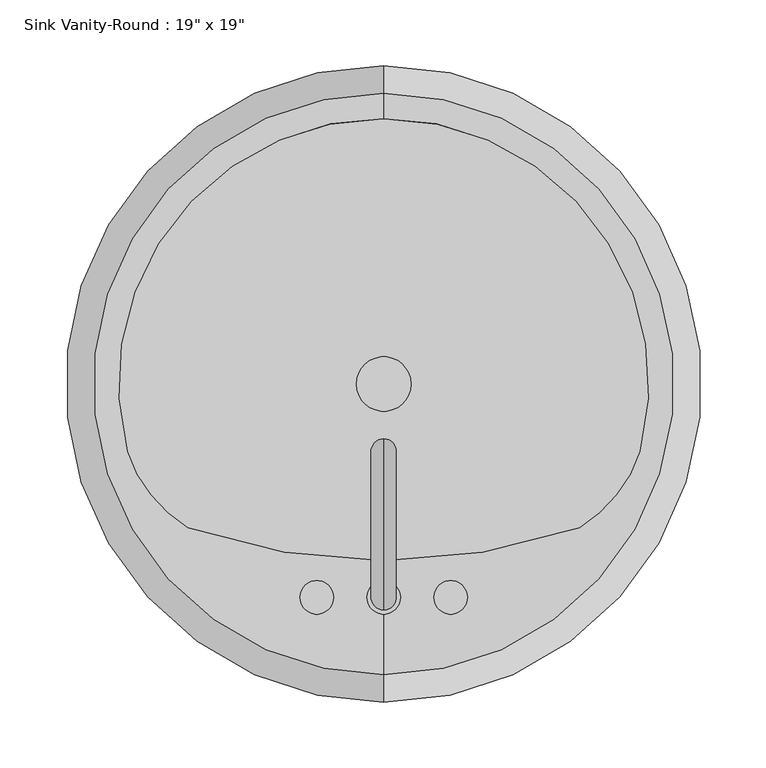
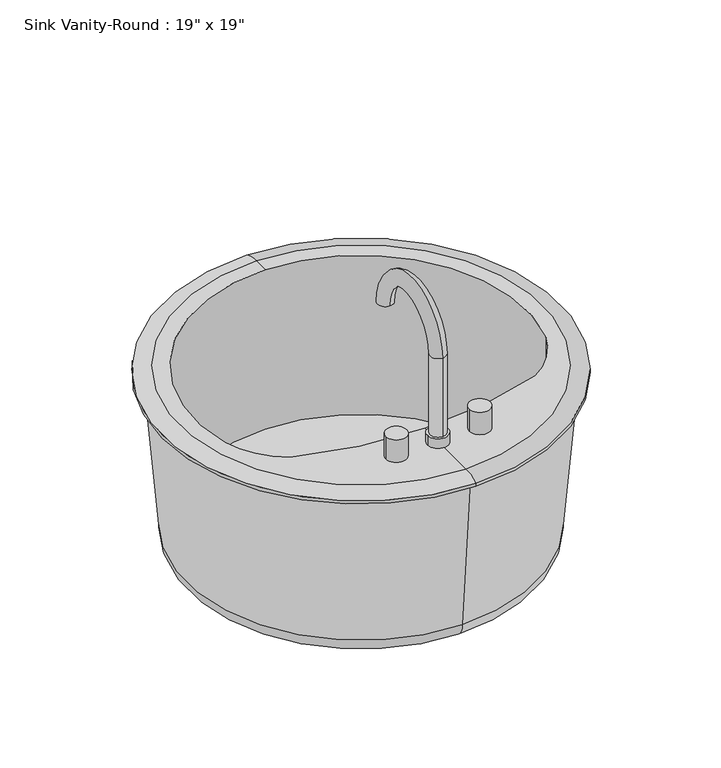
"""IFC4 building model written with IfcOpenShell, lengths in millimetres: flow terminal geometry."""

from ifc_helpers import new_model, si_unit, point, frame, frame_2d, origin, place, context, project, spatial, polyline, circle_curve, ellipse_curve, trimmed, segment, composite_curve, outline, extrude, source, transform, mapped, element, save
from ifc_brep_helpers import plane_surface, cylinder_surface, revolved_surface, advanced_brep


def flow_terminal_951b6bfb(model_context):
    return source(origin(), model_context, "Body", "SolidModel", [
        advanced_brep(
        [(83.9517406, -247.0927185, 796.925), (109.3517406, -247.0927185, 796.925), (96.6517406, -237.5677185, 909.6375), (96.6517406, -237.5677185, 809.1602909), (96.6517406, -256.6177185, 809.1602909), (96.6517406, -256.6177185, 909.6375), (96.6517406, -145.7775038, 909.6375), (96.6517406, -126.7275038, 909.6375), (83.9517406, -247.0927185, 809.1602909), (109.3517406, -247.0927185, 809.1602909)],
        [
            (0, 1, circle_curve(frame((96.6517406, -247.0927185, 796.925), z_axis=(0.0, 0.0, -1.0), x_axis=(1.0, 0.0, 0.0)), 12.7)),
            (1, 0, circle_curve(frame((96.6517406, -247.0927185, 796.925), z_axis=(0.0, 0.0, -1.0), x_axis=(1.0, 0.0, 0.0)), 12.7)),
            (2, 3),
            (3, 4, circle_curve(frame((96.6517406, -247.0927185, 809.1602909), z_axis=(0.0, 0.0, 1.0), x_axis=(0.0, -1.0, 0.0)), 9.525)),
            (4, 5),
            (5, 2, circle_curve(frame((96.6517406, -247.0927185, 909.6375), z_axis=(0.0, 0.0, -1.0), x_axis=(0.0, -1.0, 0.0)), 9.525)),
            (4, 3, circle_curve(frame((96.6517406, -247.0927185, 809.1602909), z_axis=(0.0, 0.0, 1.0), x_axis=(0.0, -1.0, 0.0)), 9.525)),
            (2, 5, circle_curve(frame((96.6517406, -247.0927185, 909.6375), z_axis=(0.0, 0.0, -1.0), x_axis=(0.0, -1.0, 0.0)), 9.525)),
            (6, 7, circle_curve(frame((96.6517406, -136.2525038, 909.6375), z_axis=(0.0, 0.0, -1.0), x_axis=(0.0, 1.0, 0.0)), 9.525)),
            (7, 6, circle_curve(frame((96.6517406, -136.2525038, 909.6375), z_axis=(0.0, 0.0, -1.0), x_axis=(0.0, 1.0, 0.0)), 9.525)),
            (5, 7, circle_curve(frame((96.6517406, -191.6726112, 909.6375), z_axis=(-1.0, 0.0, 0.0), x_axis=(0.0, -1.0, 0.0)), 64.9451073)),
            (6, 2, circle_curve(frame((96.6517406, -191.6726112, 909.6375), z_axis=(1.0, 0.0, 0.0), x_axis=(0.0, -1.0, 0.0)), 45.8951073)),
            (8, 9, circle_curve(frame((96.6517406, -247.0927185, 809.1602909), z_axis=(0.0, 0.0, 1.0), x_axis=(1.0, 0.0, 0.0)), 12.7)),
            (9, 8, circle_curve(frame((96.6517406, -247.0927185, 809.1602909), z_axis=(0.0, 0.0, 1.0), x_axis=(1.0, 0.0, 0.0)), 12.7)),
            (9, 1),
            (0, 8),
        ],
        [
            plane_surface(frame((96.6517406, -237.5677185, 796.925), z_axis=(0.0, 0.0, -1.0), x_axis=(1.0, 0.0, 0.0))),
            cylinder_surface(frame((96.6517406, -247.0927185, 796.925), z_axis=(0.0, 0.0, -1.0), x_axis=(0.0, -1.0, 0.0)), 9.525),
            plane_surface(frame((96.6517406, -191.6726112, 909.6375), z_axis=(0.0, 0.0, -1.0), x_axis=(0.0, 1.0, 0.0))),
            revolved_surface(trimmed(ellipse_curve(frame((96.6517406, -247.0927185, 909.6375), z_axis=(0.0, 0.0, 1.0), x_axis=(0.0, -1.0, 0.0)), 9.525, 9.525), [point((96.6517406, -237.5677185, 909.6375))], [point((96.6517406, -256.6177185, 909.6375))], True, "CARTESIAN"), (96.6517406, -191.6726112, 909.6375), (1.0, 0.0, 0.0)),
            revolved_surface(trimmed(ellipse_curve(frame((96.6517406, -247.0927185, 909.6375), z_axis=(0.0, 0.0, 1.0), x_axis=(0.0, -1.0, 0.0)), 9.525, 9.525), [point((96.6517406, -256.6177185, 909.6375))], [point((96.6517406, -237.5677185, 909.6375))], True, "CARTESIAN"), (96.6517406, -191.6726112, 909.6375), (1.0, 0.0, 0.0)),
            plane_surface(frame((109.3517406, -247.0927185, 809.1602909), z_axis=(0.0, 0.0, 1.0), x_axis=(0.0, -1.0, 0.0))),
            cylinder_surface(frame((96.6517406, -247.0927185, 796.925), z_axis=(0.0, 0.0, 1.0), x_axis=(1.0, 0.0, 0.0)), 12.7),
        ],
        [
            (0, [[1, 2]]),
            (1, [[3, 4, 5, 6]]),
            (1, [[-5, 7, -3, 8]]),
            (2, [[9, 10]]),
            (3, [[11, -9, 12, -6]]),
            (4, [[-12, -10, -11, -8]]),
            (5, [[13, 14], [-7, -4]]),
            (6, [[15, -1, 16, -14]]),
            (6, [[-16, -2, -15, -13]]),
        ],
    ),
        extrude(outline(composite_curve([segment(trimmed(circle_curve(frame_2d((45.8517406, -247.0927185)), 12.7), [point((33.1517406, -247.0927185))], [point((58.5517406, -247.0927185))], False, "CARTESIAN"), True, "CONTINUOUS"), segment(trimmed(circle_curve(frame_2d((45.8517406, -247.0927185)), 12.7), [point((58.5517406, -247.0927185))], [point((33.1517406, -247.0927185))], False, "CARTESIAN"), True, "CONTINUOUS")], self_intersect=False)), frame((0.0, 0.0, 796.925), z_axis=(0.0, 0.0, 1.0), x_axis=(1.0, 0.0, 0.0)), (0.0, 0.0, 1.0), 28.575),
        extrude(outline(composite_curve([segment(trimmed(circle_curve(frame_2d((147.4517406, -247.0927185)), 12.7), [point((134.7517406, -247.0927185))], [point((160.1517406, -247.0927185))], False, "CARTESIAN"), True, "CONTINUOUS"), segment(trimmed(circle_curve(frame_2d((147.4517406, -247.0927185)), 12.7), [point((160.1517406, -247.0927185))], [point((134.7517406, -247.0927185))], False, "CARTESIAN"), True, "CONTINUOUS")], self_intersect=False)), frame((0.0, 0.0, 796.925), z_axis=(0.0, 0.0, 1.0), x_axis=(1.0, 0.0, 0.0)), (0.0, 0.0, 1.0), 28.575),
        extrude(outline(composite_curve([segment(trimmed(circle_curve(frame_2d((96.6517406, -85.1677185)), 20.6375), [point((76.0142406, -85.1677185))], [point((117.2892406, -85.1677185))], False, "CARTESIAN"), True, "CONTINUOUS"), segment(trimmed(circle_curve(frame_2d((96.6517406, -85.1677185)), 20.6375), [point((117.2892406, -85.1677185))], [point((76.0142406, -85.1677185))], False, "CARTESIAN"), True, "CONTINUOUS")], self_intersect=False)), frame((0.0, 0.0, 571.5), z_axis=(0.0, 0.0, 1.0), x_axis=(1.0, 0.0, 0.0)), (0.0, 0.0, 1.0), 21.1842611),
        advanced_brep(
        [(96.6517406, 135.3870093, 796.925), (96.6517406, 156.1322815, 791.36875), (96.6517406, -326.4677185, 791.36875), (96.6517406, -305.7224463, 796.925), (96.6517406, -219.2662048, 796.925), (-52.1534933, -194.0861398, 796.925), (-98.1703414, -136.2525038, 796.925), (96.6517406, 116.2405705, 796.925), (291.4738225, -136.2525038, 796.925), (245.4569744, -194.0861398, 796.925), (96.6517406, 107.1264028, 571.5), (96.6517406, -85.1677185, 571.5), (96.6517406, -277.4618398, 571.5), (96.6517406, -298.0181731, 592.6842611), (96.6517406, 127.6827361, 592.6842611), (96.6517406, -314.5614685, 787.4), (96.6517406, 144.2260315, 787.4), (96.6517406, -326.4677185, 787.4), (96.6517406, 156.1322815, 787.4), (245.4569744, -194.0861398, 592.6842611), (291.4738225, -136.2525038, 592.6842611), (-98.1703414, -136.2525038, 592.6842611), (-52.1534933, -194.0861398, 592.6842611)],
        [
            (0, 1, circle_curve(frame((96.6517406, 139.1020246, 769.289434), z_axis=(-1.0, 0.0, 0.0), x_axis=(0.0, 1.0, 0.0)), 27.8841505)),
            (1, 2, circle_curve(frame((96.6517406, -85.1677185, 791.36875), z_axis=(0.0, 0.0, 1.0), x_axis=(0.0, -1.0, 0.0)), 241.3)),
            (2, 3, circle_curve(frame((96.6517406, -309.4374616, 769.289434), z_axis=(-1.0, 0.0, 0.0), x_axis=(0.0, -1.0, 0.0)), 27.8841505)),
            (3, 0, circle_curve(frame((96.6517406, -85.1677185, 796.925), z_axis=(0.0, 0.0, -1.0), x_axis=(0.0, -1.0, 0.0)), 220.5547278)),
            (2, 1, circle_curve(frame((96.6517406, -85.1677185, 791.36875), z_axis=(0.0, 0.0, 1.0), x_axis=(0.0, -1.0, 0.0)), 241.3)),
            (0, 3, circle_curve(frame((96.6517406, -85.1677185, 796.925), z_axis=(0.0, 0.0, -1.0), x_axis=(0.0, -1.0, 0.0)), 220.5547278)),
            (3, 4),
            (4, 5, circle_curve(frame((96.6517406, 233.0168462, 796.925), z_axis=(0.0, 0.0, -1.0), x_axis=(1.0, 0.0, 0.0)), 452.283051)),
            (5, 6, circle_curve(frame((1.3689689, -104.2755165, 796.925), z_axis=(0.0, 0.0, -1.0), x_axis=(1.0, 0.0, 0.0)), 104.5495194)),
            (6, 7, circle_curve(frame((96.6517406, -85.1677185, 796.925), z_axis=(0.0, 0.0, -1.0), x_axis=(1.0, 0.0, 0.0)), 201.408289)),
            (7, 0),
            (7, 8, circle_curve(frame((96.6517406, -85.1677185, 796.925), z_axis=(0.0, 0.0, -1.0), x_axis=(1.0, 0.0, 0.0)), 201.408289)),
            (8, 9, circle_curve(frame((191.9345122, -104.2755165, 796.925), z_axis=(0.0, 0.0, -1.0), x_axis=(1.0, 0.0, 0.0)), 104.5495194)),
            (9, 4, circle_curve(frame((96.6517406, 233.0168462, 796.925), z_axis=(0.0, 0.0, -1.0), x_axis=(1.0, 0.0, 0.0)), 452.283051)),
            (10, 11),
            (11, 12),
            (12, 10, circle_curve(frame((96.6517406, -85.1677185, 571.5), z_axis=(0.0, 0.0, -1.0), x_axis=(0.0, -1.0, 0.0)), 192.2941213)),
            (10, 12, circle_curve(frame((96.6517406, -85.1677185, 571.5), z_axis=(0.0, 0.0, -1.0), x_axis=(0.0, -1.0, 0.0)), 192.2941213)),
            (12, 13, circle_curve(frame((96.6517406, -277.4618398, 592.0656396), z_axis=(-1.0, 0.0, 0.0), x_axis=(0.0, -1.0, 0.0)), 20.5656396)),
            (13, 14, circle_curve(frame((96.6517406, -85.1677185, 592.6842611), z_axis=(0.0, 0.0, -1.0), x_axis=(0.0, -1.0, 0.0)), 212.8504546)),
            (14, 10, circle_curve(frame((96.6517406, 107.1264028, 592.0656396), z_axis=(-1.0, 0.0, 0.0), x_axis=(0.0, 1.0, 0.0)), 20.5656396)),
            (14, 13, circle_curve(frame((96.6517406, -85.1677185, 592.6842611), z_axis=(0.0, 0.0, -1.0), x_axis=(0.0, -1.0, 0.0)), 212.8504546)),
            (13, 15),
            (15, 16, circle_curve(frame((96.6517406, -85.1677185, 787.4), z_axis=(0.0, 0.0, -1.0), x_axis=(0.0, -1.0, 0.0)), 229.39375)),
            (16, 14),
            (16, 15, circle_curve(frame((96.6517406, -85.1677185, 787.4), z_axis=(0.0, 0.0, -1.0), x_axis=(0.0, -1.0, 0.0)), 229.39375)),
            (15, 17),
            (17, 18, circle_curve(frame((96.6517406, -85.1677185, 787.4), z_axis=(0.0, 0.0, -1.0), x_axis=(0.0, -1.0, 0.0)), 241.3)),
            (18, 16),
            (18, 17, circle_curve(frame((96.6517406, -85.1677185, 787.4), z_axis=(0.0, 0.0, -1.0), x_axis=(0.0, -1.0, 0.0)), 241.3)),
            (1, 18),
            (17, 2),
            (19, 20, circle_curve(frame((191.9345122, -104.2755165, 592.6842611), z_axis=(0.0, 0.0, 1.0), x_axis=(1.0, 0.0, 0.0)), 104.5495194)),
            (20, 21, circle_curve(frame((96.6517406, -85.1677185, 592.6842611), z_axis=(0.0, 0.0, 1.0), x_axis=(1.0, 0.0, 0.0)), 201.408289)),
            (21, 22, circle_curve(frame((1.3689689, -104.2755165, 592.6842611), z_axis=(0.0, 0.0, 1.0), x_axis=(1.0, 0.0, 0.0)), 104.5495194)),
            (22, 19, circle_curve(frame((96.6517406, 233.0168462, 592.6842611), z_axis=(0.0, 0.0, 1.0), x_axis=(1.0, 0.0, 0.0)), 452.283051)),
            (22, 5),
            (9, 19),
            (21, 6),
            (20, 8),
        ],
        [
            revolved_surface(trimmed(ellipse_curve(frame((96.6517406, -309.4374616, 769.289434), z_axis=(-1.0, 0.0, 0.0), x_axis=(0.0, -1.0, 0.0)), 27.8841505, 27.8841505), [point((96.6517406, -326.4677185, 791.36875))], [point((96.6517406, -305.7224463, 796.925))], True, "CARTESIAN"), (96.6517406, -85.1677185, 796.925), (0.0, 0.0, 1.0)),
            plane_surface(frame((96.6517406, -85.1677185, 796.925), z_axis=(0.0, 0.0, 1.0), x_axis=(0.0, -1.0, 0.0))),
            plane_surface(frame((96.6517406, -85.1677185, 571.5), z_axis=(0.0, 0.0, -1.0), x_axis=(0.0, -1.0, 0.0))),
            revolved_surface(trimmed(ellipse_curve(frame((96.6517406, -277.4618398, 592.0656396), z_axis=(-1.0, 0.0, 0.0), x_axis=(0.0, -1.0, 0.0)), 20.5656396, 20.5656396), [point((96.6517406, -277.4618398, 571.5))], [point((96.6517406, -298.0181731, 592.6842611))], True, "CARTESIAN"), (96.6517406, -85.1677185, 796.925), (0.0, 0.0, 1.0)),
            revolved_surface(polyline([(96.6517406, -298.0181731, 592.6842611), (96.6517406, -314.5614685, 787.4)]), (96.6517406, -85.1677185, 796.925), (0.0, 0.0, 1.0)),
            plane_surface(frame((96.6517406, -85.1677185, 787.4), z_axis=(0.0, 0.0, -1.0), x_axis=(0.0, -1.0, 0.0))),
            cylinder_surface(frame((96.6517406, -85.1677185, 796.925), z_axis=(0.0, 0.0, 1.0), x_axis=(0.0, -1.0, 0.0)), 241.3),
            plane_surface(frame((548.9347916, 233.0168462, 592.6842611), z_axis=(0.0, 0.0, 1.0), x_axis=(0.0, 1.0, 0.0))),
            revolved_surface(polyline([(548.9347916, 233.0168462, 796.925), (548.9347916, 233.0168462, 592.6842611)]), (96.6517406, 233.0168462, 592.6842611), (0.0, 0.0, 1.0)),
            revolved_surface(polyline([(105.91848829999999, -104.2755165, 796.925), (105.91848829999999, -104.2755165, 592.6842611)]), (1.3689689, -104.2755165, 592.6842611), (0.0, 0.0, 1.0)),
            revolved_surface(polyline([(298.0600296, -85.1677185, 796.925), (298.0600296, -85.1677185, 592.6842611)]), (96.6517406, -85.1677185, 592.6842611), (0.0, 0.0, 1.0)),
            revolved_surface(polyline([(296.4840316, -104.2755165, 796.925), (296.4840316, -104.2755165, 592.6842611)]), (191.9345122, -104.2755165, 592.6842611), (0.0, 0.0, 1.0)),
        ],
        [
            (0, [[1, 2, 3, 4]]),
            (0, [[5, -1, 6, -3]]),
            (1, [[7, 8, 9, 10, 11, -4]]),
            (1, [[-11, 12, 13, 14, -7, -6]]),
            (2, [[15, 16, 17]]),
            (2, [[-15, 18, -16]]),
            (3, [[19, 20, 21, -17]]),
            (3, [[-21, 22, -19, -18]]),
            (4, [[23, 24, 25, -20]]),
            (4, [[-25, 26, -23, -22]]),
            (5, [[27, 28, 29, -24]]),
            (5, [[-29, 30, -27, -26]]),
            (6, [[31, -28, 32, -2]]),
            (6, [[-32, -30, -31, -5]]),
            (7, [[33, 34, 35, 36]]),
            (8, [[37, -8, -14, 38, -36]]),
            (9, [[39, -9, -37, -35]]),
            (10, [[40, -12, -10, -39, -34]]),
            (11, [[-38, -13, -40, -33]]),
        ],
    ),
    ])


if __name__ == "__main__":
    model = new_model("IFC4")
    model_context = context("Model", 3, world=origin())
    ifc_project = project(units=[si_unit("LENGTHUNIT", "METRE", prefix="MILLI")], contexts=[model_context])
    site = spatial("IfcSite", under=ifc_project)
    building = spatial("IfcBuilding", under=site)
    placement = place(None, origin())
    flow_terminal_shape = flow_terminal_951b6bfb(model_context)
    element("IfcFlowTerminal", 1, ObjectType="Sink Vanity-Round : 19\" x 19\"", at=placement, inside=building, context=model_context, shape_type="MappedRepresentation", body=[
        mapped(flow_terminal_shape, transform((0.0, 0.0, 0.0), x_axis=(1.0, 0.0, 0.0), y_axis=(0.0, 1.0, 0.0), z_axis=(0.0, 0.0, 1.0))),
    ])
    save(model, "model.ifc")

# Revit data of these elements
# Type "Sink Vanity-Round : 19\" x 19\""
#   Assembly Code = "D2010400"
#   Top Of Counter = 2' - 7"
#   Basin Material = Porcelain, Linen
#   Faucet Material = Steel, Polished
#   Default Elevation = 0
# Element 1 (IfcFlowTerminal, "Sink Vanity-Round : 19\" x 19\"")
#   Materials on its faces: "Porcelain, Linen", "Steel, Polished"
# Materials
#   "Porcelain, Linen": class "Ceramic", colour RGB 249 239 230, transparency 0, Description = "Porcelain, linen", Cost = 0
#   "Steel, Polished": class "Metal", colour RGB 57 57 57, transparency 0, Description = "Polished steel", Cost = 0
